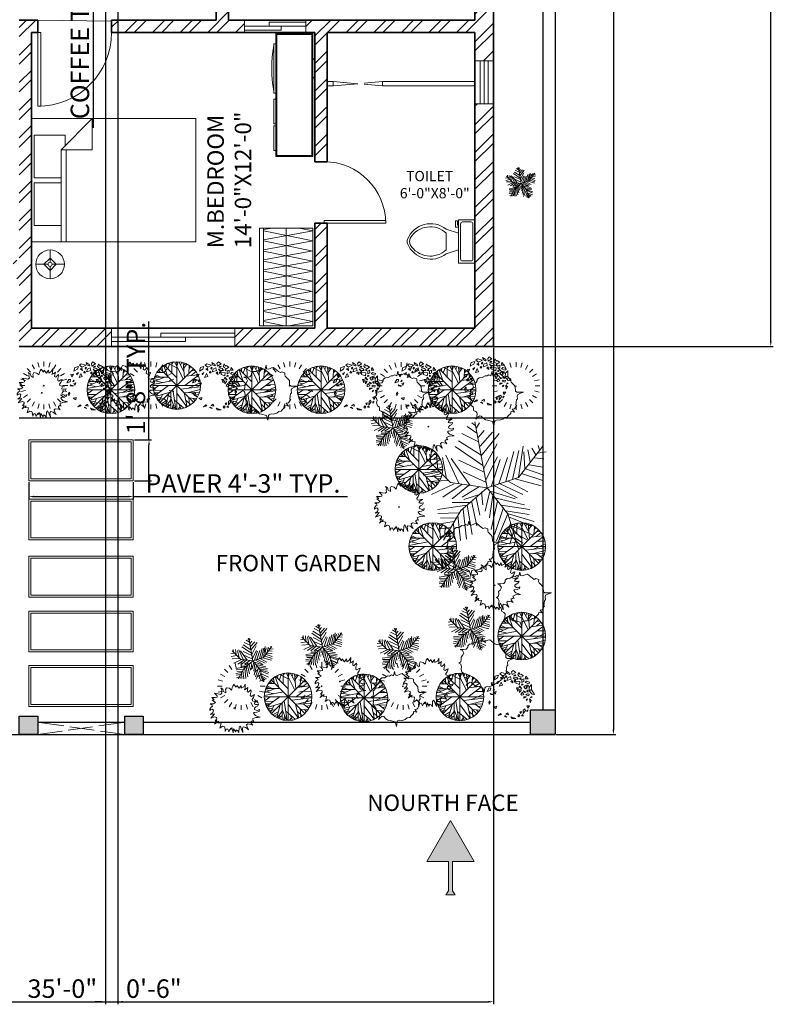
# Model space of a CAD drawing. Units: inches. Extents: x 889 to 1572, y 7262 to 8387.
# Tile 2 of 8: x 1205 to 1572, y 7262 to 7742. Entities that reach past the tile are written whole.
import ezdxf

# ---------------------------------------------------------------- set-up
doc = ezdxf.new("R2010")
doc.units = ezdxf.units.IN
doc.linetypes.add('ACAD_ISO02W100', pattern=[15, 12, -3])
for name, color, linetype, lineweight in [('A-ANNO-DIMS', 2, 'Continuous', 18), ('A-ANNO-SYMB', 7, 'Continuous', 18), ('A-ANNO-TEXT', 7, 'Continuous', 18), ('A-AREA-IDEN', 7, 'Continuous', 18), ('A-DOOR', 4, 'Continuous', 18), ('A-FIXT-HIDN', 9, 'ACAD_ISO02W100', 13), ('A-FLOR-FIXT', 9, 'Continuous', 18), ('A-FURN', 8, 'Continuous', 18), ('A-FURN-PATT', 252, 'Continuous', 13), ('A-WALL', 7, 'Continuous', 35), ('A-WALL-PATT', 252, 'Continuous', 13), ('C-SITE', 7, 'Continuous', 30), ('C-SITE-PATT', 252, 'Continuous', 13), ('L-PLNT', 94, 'Continuous', 13), ('L-PVMT', 8, 'Continuous', 18)]:
    doc.layers.add(name, color=color, linetype=linetype, lineweight=lineweight)
doc.layers.add('A-GLAZ', color=244, linetype='Continuous', lineweight=18, true_color=0x991b1e)
doc.layers.add('C-SITE-GATE', color=244, linetype='ACAD_ISO02W100', lineweight=18, true_color=0x991b1e)
doc.styles.get("Standard").update_dxf_attribs({"font": 'arial.ttf'})
doc.dimstyles.new('ISO-25', dxfattribs={"dimtxt": 9, "dimasz": 2.5, "dimexe": 1.25, "dimexo": 0.625, "dimtad": 1, "dimlunit": 3, "dimtxsty": 'Standard', "dimcen": 2.5, "dimadec": 0, "dimazin": 0, "dimtfac": 1, "dimtmove": 0, "dimatfit": 3, "dimfxl": 1, "dimarcsym": 0})

# ---------------------------------------------------------------- blocks, each defined once
blk = doc.blocks.new('*U3')
for p, q in [((0, 0), (0, -6)), ((-40, 0), (-40, -6))]:
    blk.add_line(p, q)
blk.add_lwpolyline([(0, 0), (0, 40), (-1.75, 40), (-1.75, 0)], close=True)
blk.add_arc((0, 0), 40, 90, 180)
blk = doc.blocks.new('*U4')
for p, q in [((0, 0), (0, 6)), ((40, 0), (40, 6))]:
    blk.add_line(p, q)
blk.add_lwpolyline([(0, 0), (0, -40), (1.75, -40), (1.75, 0)], close=True)
blk.add_arc((0, 0), 40, 270, 0)
blk = doc.blocks.new('*U10')
for p, q in [((9.5, -6), (9.5, -2)), ((-10, -8.5), (-8, -8.5)), ((-10, -9.5), (-10, -8.5)), ((-7, -9.5), (-10, -9.5)), ((-8, -8.5), (-8, -8)), ((-7, -8), (-7, -9.5)), ((-4, -8), (-6, -14)), ((4, -8), (6, -14)), ((4, -14), (-4, -14))]:
    blk.add_line(p, q)
blk.add_lwpolyline([(10.5, -8), (10.5, 0), (-10.5, 0), (-10.5, -8)], close=True)
for points in [[(-9.5, -2), (-9.5, -6)], [(8.5, -1), (-8.5, -1)], [(-8.5, -7), (8.5, -7)]]:
    blk.add_lwpolyline(points)
for centre, radius, start, end in [((-8.62, -1.88), 0.884, 81.8699, 188.1301), ((8.62, -1.88), 0.884, 351.8699, 98.1301), ((-8.62, -6.12), 0.884, 171.8699, 278.1301), ((8.62, -6.12), 0.884, 261.8699, 8.1301), ((3.52, -21.58), 12.17, 141.4691, 247.9714), ((4.2, -21.82), 11.33, 136.3677, 238.9468), ((-3.52, -21.58), 12.17, 292.0284, 38.5307), ((-4.2, -21.82), 11.33, 301.053, 43.6321), ((0, -27.88), 4, 245.7318, 294.2682), ((0, -29), 4, 254.8605, 285.1395)]:
    blk.add_arc(centre, radius, start, end)
blk = doc.blocks.new('Bed - Queen')
for p, q in [((0, -80.00003), (0, 0)), ((0, 0), (59.99999, 0)), ((59.99999, 0), (59.99999, -80.00003)), ((7.99999, -1.2), (28.79998, -1.2)), ((7.99999, -14.4), (7.99999, -1.2)), ((28.79998, -1.2), (28.79998, -14.4)), ((31.19999, -1.2), (51.99999, -1.2)), ((31.19999, -14.4), (31.19999, -1.2)), ((51.99999, -1.2), (51.99999, -16.4)), ((0, -14.4), (44.8, -14.4)), ((44.8, -16.8), (0, -16.8)), ((59.99999, -29.6), (44.8, -14.4)), ((44.8, -14.4), (44.8, -29.6)), ((51.99999, -16.4), (46.79936, -16.4)), ((44.8, -29.6), (59.99999, -29.6)), ((59.99999, -80.00003), (0, -80.00003))]:
    blk.add_line(p, q)
blk = doc.blocks.new('Entertainment Center')
for p, q in [((-4, 0), (-5, -1)), ((4, 0), (-4, 0)), ((5, -1), (4, 0)), ((-17, -19), (-17, -1)), ((-17, -1), (43, -1)), ((-16.5, -18.5), (-16.5, -1.5)), ((-16.5, -1.5), (42.5, -1.5)), ((42.5, -1.5), (42.5, -18.5)), ((43, -1), (43, -19)), ((43, -19), (-17, -19)), ((42.5, -18.5), (-16.5, -18.5)), ((-12, -20), (-12, -19)), ((12, -19), (12, -20)), ((15, -20), (15, -19)), ((27, -19), (27, -20)), ((28, -20), (28, -19)), ((40, -19), (40, -20)), ((12, -20), (-12, -20)), ((27, -20), (15, -20)), ((40, -20), (28, -20))]:
    blk.add_line(p, q)
blk.add_arc((0, 40), 61, 259.6111, 280.3889)
blk = doc.blocks.new('*U15')
for p, q in [((-8.737, 47.138), (-17.069, 52.711)), ((-10.186, 53.64), (-13.084, 55.962)), ((0, 0), (-10.5, 57)), ((-9.099, 51.782), (-6.563, 55.962)), ((-7.288, 39.707), (-21.778, 46.673)), ((-7.65, 43.423), (-2.578, 49.46)), ((-5.839, 35.992), (4.667, 48.067)), ((-5.114, 27.632), (10.463, 46.673)), ((-3.665, 19.273), (-27.574, 35.527)), ((-5.114, 28.097), (-24.676, 40.636)), ((-2.941, 16.486), (8.652, 37.85)), ((27, 9), (48, 36)), ((27.127, 9.056), (31.112, 35.992)), ((38.719, 34.134), (41.979, 28.561)), ((44.153, 36.456), (45.239, 32.741)), ((-31.5, 4.5), (-52.5, 25.5)), ((-48.585, 21.131), (-49.309, 29.026)), ((-43.513, 28.561), (-42.427, 15.558)), ((-38.442, 26.239), (-34.819, 7.663)), ((-35.544, 28.097), (-24.314, 3.947)), ((-1.129, 6.734), (9.014, 26.704)), ((10.101, 3.483), (17.708, 26.239)), ((16.259, 5.805), (23.142, 31.348)), ((22.055, 7.198), (27.489, 32.277)), ((31.836, 30.883), (32.561, 16.486)), ((35.096, 32.741), (37.27, 22.524)), ((40.53, 25.775), (48.862, 24.846)), ((43.791, 29.954), (51.036, 30.883)), ((-47.498, 19.737), (-55.83, 18.344)), ((-14.533, 2.09), (-30.834, 25.31)), ((-24.314, 23.917), (-2.941, 13.7)), ((3.942, 1.625), (11.187, 24.381)), ((36.183, 19.737), (48.137, 17.88)), ((-40.615, 13.7), (-55.105, 10.913)), ((-20.691, 13.7), (-1.129, 4.876)), ((0, 0), (27, 9)), ((29.662, 12.307), (48.137, 6.269)), ((33.285, 16.486), (48.862, 10.913)), ((-33.37, 6.269), (-52.207, 5.34)), ((-28.299, 3.483), (-47.86, -5.805)), ((-21.416, 3.018), (-38.079, -8.128)), ((0, 0), (-31.5, 4.5)), ((-15.982, 2.09), (-30.11, -9.521)), ((0, 0), (-22.5, -19.5)), ((-6.563, 1.161), (-21.416, -8.128)), ((0, 0), (18, -22.5)), ((6.478, 1.625), (26.04, -8.592)), ((11.187, 3.483), (30.749, -5.805)), ((18.07, 5.805), (35.096, -3.483)), ((24.229, 7.663), (46.688, 1.625)), ((-6.563, -5.805), (-19.967, -9.985)), ((-4.752, -3.483), (-3.665, -14.629)), ((2.493, -3.019), (-1.491, -20.202)), ((1.769, -2.555), (24.229, -9.521)), ((5.029, -6.27), (2.131, -25.775)), ((-17.431, -15.094), (-42.789, -18.809)), ((-15.257, -12.772), (-30.11, -12.772)), ((-17.069, -15.094), (-12.721, -40.172)), ((-13.446, -11.378), (-8.737, -32.741)), ((-9.461, -8.592), (-6.201, -23.453)), ((9.014, -11.378), (3.58, -35.992)), ((14.085, -16.951), (6.478, -40.172)), ((7.565, -9.056), (32.198, -14.629)), ((12.274, -15.094), (36.907, -18.809)), ((-24.314, -21.596), (-42.427, -22.06)), ((-22.5, -19.5), (-37.5, -45)), ((-25.038, -23.918), (-22.865, -45.281)), ((-20.691, -18.345), (-17.793, -44.352)), ((18.07, -22.524), (8.289, -45.745)), ((16.259, -19.738), (36.183, -22.989)), ((18, -22.5), (27, -52.5)), ((18.433, -22.524), (40.53, -29.026)), ((19.157, -25.311), (38.719, -33.206)), ((-28.299, -29.026), (-42.789, -31.348)), ((-26.849, -26.24), (-40.253, -25.775)), ((-29.023, -30.884), (-27.936, -43.887)), ((20.244, -30.419), (15.897, -44.816)), ((21.331, -32.741), (39.081, -40.636)), ((-30.834, -34.135), (-42.427, -35.528)), ((-34.457, -39.708), (-40.978, -42.494)), ((-32.646, -36.921), (-31.921, -44.352)), ((22.78, -37.85), (19.519, -48.532)), ((22.78, -38.314), (34.372, -44.816)), ((24.591, -45.745), (23.142, -50.854)), ((24.591, -43.423), (30.749, -47.603)), ((26.764, -49.925), (28.213, -50.854))]:
    blk.add_line(p, q)
blk = doc.blocks.new('*U14')
for points in [[(-5.78, 9.75), (-7.54, 9.23), (-8.01, 7.5), (-6.26, 8.45)], [(-4.43, 11.05), (-5.18, 10.36), (-3.96, 9.49), (-2.07, 10.36)], [(-2, 11.66), (-1.6, 10.62), (-0.52, 10.1), (-0.18, 10.62), (-0.79, 10.96)], [(1.24, 12), (0.56, 11.31), (0.76, 10.01), (2.52, 11.05)], [(2.59, 9.93), (1.84, 9.75), (1.64, 9.23), (2.32, 9.41)], [(4.14, 11.14), (3.6, 10.01), (4, 9.23), (5.22, 8.71), (6.3, 9.41), (5.08, 10.19), (4.61, 10.01)], [(-8.14, 6.03), (-9.36, 5.95), (-9.02, 4.73)], [(-5.78, 6.81), (-6.66, 6.21), (-6.52, 5.69)], [(-4.57, 6.38), (-5.45, 4.47), (-3.89, 4.82)], [(-4.84, 8.63), (-3.83, 7.85), (-4.03, 8.97)], [(-2.88, 7.5), (-3.15, 6.64), (-2.27, 6.72)], [(-1.94, 9.49), (-2.48, 8.97), (-2.27, 8.54), (-1.8, 9.06)], [(0.02, 9.06), (-1.33, 8.54), (-1.73, 7.16), (0.29, 7.76)], [(0.76, 7.16), (0.09, 6.46), (1.1, 5.95)], [(1.37, 8.54), (3.13, 8.8), (3.8, 7.85), (1.91, 7.76)], [(1.71, 6.29), (1.71, 7.07), (2.65, 7.5), (2.11, 6.9)], [(2.52, 6.81), (2.52, 5.86), (4.41, 5.17), (4.61, 6.72)], [(4.61, 8.28), (4.54, 7.76), (4.95, 7.59), (4.95, 8.28)], [(5.49, 5.51), (5.42, 4.82), (6.16, 5.08)], [(6.43, 7.94), (5.49, 7.68), (5.56, 6.21), (6.5, 6.64)], [(8.12, 4.99), (7.11, 4.65), (6.5, 4.13), (7.38, 3.09), (8.12, 3.52), (7.65, 3.87)], [(7.45, 9.32), (7.11, 7.94), (8.52, 7.94)], [(7.85, 6.81), (7.18, 6.21), (9, 5.51), (9.33, 6.38)], [(10.28, 5.17), (9.2, 4.04), (9, 2.31), (10.48, 0.49), (11.76, 0.41), (10.35, 2.48), (9.33, 2.4), (10.28, 2.83)], [(-11.32, 1.79), (-9.83, 2.31), (-9.63, 3.44), (-10.44, 3.52)], [(-8.21, 0.41), (-9.43, 0.32), (-9.83, 0.84)], [(-8.21, 3.09), (-8.48, 2.31), (-7.87, 2.57)], [(-7, 1.79), (-7.94, 1.53), (-7.47, 0.49)], [(3.53, 1.88), (2.86, 3.52), (3.8, 3.52)], [(4.41, 4.56), (4.27, 3.7), (5.49, 3.26)], [(4.27, 2.74), (5.29, 2.66), (4.41, 1.27)], [(5.83, 1.53), (5.02, 0.41), (5.49, -0.02), (6.5, 0.41)], [(7.51, 1.71), (6.91, 1.27), (6.23, 2.14)], [(8.12, 0.75), (7.51, 0.15), (8.93, -0.28), (9.13, 0.49)], [(8.19, 2.57), (7.92, 2.05), (8.66, 1.53)], [(8.73, 4.73), (8.19, 4.56), (8.39, 3.87), (8.59, 4.04)], [(-10.03, -2.71), (-10.64, -3.31), (-10.44, -4.44), (-9.9, -3.49)], [(7.78, -0.8), (6.43, -1.5), (6.43, -0.72)], [(8.32, -1.75), (7.98, -2.53), (7.58, -2.1)], [(9.33, -1.75), (9.54, -3.74), (10.14, -2.53)], [(10.08, -0.63), (9.74, -1.32), (10.48, -0.89)], [(-8.28, -5.73), (-6.79, -5.3), (-7, -6.51)], [(-4.84, -8.85), (-4.43, -9.45), (-5.99, -9.8)], [(-2.34, -9.2), (-1.26, -8.5), (-0.99, -9.54)], [(4.07, -9.45), (3.53, -9.97), (4.07, -10.58), (4.61, -9.89)], [(5.29, -7.98), (4.61, -8.16), (5.02, -8.94)], [(6.03, -9.45), (5.42, -9.97), (6.16, -10.15)], [(6.1, -8.94), (6.16, -7.21), (6.91, -6.69), (7.24, -7.38)], [(8.05, -8.07), (8.59, -7.12), (7.92, -7.55)], [(9.33, -5.13), (8.46, -6.25), (7.98, -5.22)], [(-2.54, -10.06), (-3.02, -10.23), (-1.8, -10.67)], [(0.22, -10.58), (0.83, -11.27), (2.59, -11.36)]]:
    blk.add_lwpolyline(points, close=True)
blk = doc.blocks.new('*U16')
for p, q in [((-25.024, 42.079), (-31.077, 52.563)), ((-13.435, 46.72), (-16.606, 58.557)), ((-1.077, 60.601), (-1.077, 48.601)), ((11.28, 46.72), (14.452, 58.557)), ((22.87, 42.079), (28.923, 52.563)), ((-42.564, 24.554), (-53.039, 30.601)), ((-34.93, 34.454), (-43.503, 43.028)), ((32.776, 34.454), (41.349, 43.028)), ((40.409, 24.554), (50.884, 30.601)), ((-61.077, 0.601), (-49.077, 0.601)), ((-47.5, 13.04), (-59.033, 16.131)), ((45.346, 13.04), (56.878, 16.131)), ((58.923, 0.601), (46.923, 0.601)), ((-47.5, -11.837), (-59.033, -14.928)), ((-42.564, -23.351), (-53.039, -29.399)), ((40.409, -23.351), (50.884, -29.399)), ((45.346, -11.837), (56.878, -14.928)), ((-34.93, -33.251), (-43.503, -41.825)), ((-25.024, -40.876), (-31.077, -51.36)), ((-13.435, -45.517), (-16.606, -57.354)), ((-1.077, -59.399), (-1.077, -47.399)), ((11.28, -45.517), (14.452, -57.354)), ((22.87, -40.876), (28.923, -51.36)), ((32.776, -33.251), (41.349, -41.825))]:
    blk.add_line(p, q)
blk.add_lwpolyline([(-1.908, 0.978), (-2.67, -0.978), (0, 0)], close=True)
blk = doc.blocks.new('*U17')
for p, q in [((-32.6092, 50.4264), (-23.2782, 23.5674)), ((-31.2008, 51.1035), (-0.2149, 20.1818)), ((-26.4472, 46.5894), (-26.2712, 53.8116)), ((-22.0458, 42.0753), (-16.5881, 57.6486)), ((-21.1656, 55.8436), (-0.0388, 45.0094)), ((-12.5388, 54.9406), (-7.9613, 59.4546)), ((-12.3627, 32.1443), (-12.5388, 58.7776)), ((-5.3205, 59.6806), (16.5105, 16.7963)), ((2.426, 54.9406), (-1.4472, 59.9056)), ((0, 59.9996), (0, -60)), ((0.4894, 48.6208), (3.6584, 59.6806)), ((18.2711, 35.5298), (5.419, 59.6806)), ((9.8203, 51.5549), (12.8133, 58.5516)), ((19.6795, 19.5047), (16.3344, 57.6486)), ((17.0387, 51.1035), (23.2006, 55.1666)), ((17.7429, 43.6552), (25.4894, 54.2636)), ((31.6513, 50.8778), (30.2429, 30.5643)), ((-53.2078, 27.4044), (-40.1797, 20.859)), ((-49.8627, 32.8214), (-32.7853, 32.8214)), ((-45.8134, 38.2383), (-40.5318, 33.0471)), ((-43.8768, 36.4326), (-44.405, 40.2696)), ((42, 42), (-42, -42)), ((42, -42), (-42, 42)), ((-40.1797, 44.558), (-36.4825, 43.2038)), ((-37.0107, 47.0408), (-35.25, 35.5298)), ((54.3626, 25.3731), (20.9119, 0.3198)), ((23.3767, 23.3417), (53.3063, 27.4044)), ((31.1232, 42.5267), (35.8767, 48.1693)), ((36.2288, 25.1474), (48.9049, 35.0784)), ((37.1091, 37.1098), (46.6161, 37.5612)), ((-59.7219, 2.8025), (-12.0106, 12.0565)), ((-32.2571, 20.6333), (-59.1937, 9.348)), ((-58.6656, 12.7336), (-35.9543, 7.5424)), ((-57.081, 17.9248), (-47.0458, 14.7649)), ((-56.0247, 20.859), (-20.8134, 20.859)), ((-54.7923, 24.4702), (-47.75, 21.0847)), ((-54.6162, -24.7335), (-20.2853, 0.0941)), ((29.3626, -6.6771), (59.4682, 7.091)), ((38.5175, 13.4107), (58.2359, 13.6364)), ((-60, 0), (60, 0)), ((-59.7219, -4.8714), (-54.2641, -6.6771)), ((-45.2853, -0.1316), (-59.0177, -10.0627)), ((-58.4895, -12.3197), (-36.4825, -11.6426)), ((-57.081, -18.4138), (-45.2853, -17.9624)), ((-52.6797, -18.188), (-55.4966, -22.0251)), ((-53.2078, -27.442), (-16.7641, -16.6081)), ((-47.2219, -19.3166), (-50.2148, -26.3135)), ((-35.9543, -22.4765), (-44.0529, -40.5329)), ((-19.9331, -20.2194), (-28.5599, -52.721)), ((-14.8275, -15.0282), (-14.6515, -57.6865)), ((-10.074, -10.0627), (-2.5036, -59.7178)), ((-0.0388, -19.0909), (25.8415, -53.8495)), ((9.2922, -9.1598), (59.6443, -2.8401)), ((18.6232, -18.6394), (26.7218, -53.3981)), ((18.7992, -18.6394), (57.3556, -17.2853)), ((26.3697, -18.4138), (58.9401, -9.8369)), ((38.1654, -18.188), (52.426, -29.0219)), ((45.9119, -24.0564), (55.595, -22.2508)), ((-38.9472, -29.0219), (-51.4472, -30.6018)), ((-46.5177, -30.1504), (-49.5106, -33.536)), ((-32.4331, -32.4075), (-48.1021, -35.5674)), ((-43.7008, -34.6645), (-46.6937, -37.373)), ((-24.6867, -37.8244), (-38.7712, -45.7241)), ((-26.2712, -43.9185), (-34.7219, -48.6583)), ((-14.6515, -36.2445), (-27.6797, -52.9467)), ((-14.6515, -47.3041), (-25.0388, -54.3009)), ((-21.5177, -45.4984), (-19.9331, -56.1065)), ((-14.6515, -32.1818), (-3.912, -59.4922)), ((-8.4895, -47.5298), (-11.4825, -58.5893)), ((-6.2008, -36.2445), (17.919, -57.0094)), ((5.9471, -46.6269), (10.5246, -58.5893)), ((22.8485, -36.4702), (35.3485, -48.4326)), ((24.7852, -44.8213), (23.0246, -54.978)), ((30.419, -30.1504), (32.3556, -50.0125)), ((31.4753, -31.279), (49.6091, -33.3103)), ((41.5105, -32.6332), (46.088, -38.0501)), ((-6.3768, -52.721), (-9.3698, -58.815)), ((8.4119, -53.1724), (3.8344, -59.4922))]:
    blk.add_line(p, q)
blk.add_circle((0, 0), 60)
blk = doc.blocks.new('*U18')
blk.add_lwpolyline([(-4.577, 66.508), (-7.629, 55.26), (-12.588, 57.705), (-17.165, 54.771), (-22.124, 55.26), (-29.372, 50.859), (-36.619, 50.37), (-41.578, 45.968), (-41.578, 42.056), (-45.393, 37.655), (-52.259, 36.677), (-60.651, 36.677), (-54.929, 33.743), (-51.115, 27.385), (-54.548, 21.028), (-58.362, 17.116), (-57.599, 11.248), (-58.744, 5.379), (-63.703, 2.445), (-59.125, 0), (-56.837, -6.846), (-58.362, -13.204), (-56.455, -20.539), (-52.259, -23.473), (-51.115, -27.386), (-51.115, -32.276), (-45.011, -35.21), (-41.96, -39.122), (-42.723, -47.925), (-45.393, -54.282), (-40.434, -49.392), (-35.475, -45.969), (-31.66, -46.947), (-27.083, -51.837), (-21.361, -56.238), (-16.021, -56.727), (-3.433, -60.151), (0, -71.887), (1.526, -60.151), (3.052, -58.194), (8.392, -56.238), (14.114, -56.727), (22.506, -54.282), (27.465, -50.37), (33.95, -49.392), (37.002, -44.991), (42.723, -39.611), (43.105, -35.699), (45.012, -34.721), (51.878, -36.188), (46.157, -29.342), (51.878, -28.364), (53.785, -25.919), (56.074, -21.517), (57.6, -20.539), (55.693, -18.094), (57.219, -5.868), (59.889, -2.934), (58.744, 3.423), (60.27, 7.824), (67.137, 11.248), (74.766, 14.182), (67.899, 13.693), (58.363, 13.693), (54.93, 16.627), (54.167, 27.874), (50.353, 32.276), (43.868, 39.122), (42.723, 42.545), (43.105, 47.436), (35.476, 49.881), (31.661, 47.925), (27.084, 50.859), (14.496, 61.128), (9.155, 59.661), (2.289, 56.727), (-3.051, 57.705)], close=True)
blk = doc.blocks.new('*U19')
for points in [[(0, 60.64), (-3.051, 56.238), (-4.196, 52.815), (-5.34, 47.925), (-6.103, 45.969), (-11.062, 50.859), (-18.691, 52.326), (-20.98, 47.436), (-20.217, 43.524), (-20.598, 39.611), (-25.939, 43.035), (-27.846, 49.392), (-33.186, 52.326), (-30.516, 47.436), (-31.279, 43.035), (-30.135, 38.144), (-33.568, 35.21), (-40.815, 36.677), (-49.208, 38.144), (-46.919, 36.677), (-42.341, 31.787), (-42.341, 28.364), (-46.537, 27.386), (-55.692, 27.386), (-49.97, 22.006), (-54.548, 21.028), (-46.156, 14.671), (-51.496, 11.248), (-59.888, 11.248), (-55.692, 8.803), (-53.785, 5.38), (-57.218, 3.423), (-60.651, -1.467), (-61.033, -4.89), (-59.125, -3.423), (-54.548, -1.467), (-51.496, -4.401), (-53.022, -10.269), (-59.125, -15.16), (-49.208, -13.204), (-58.362, -24.451), (-48.445, -21.028), (-43.486, -22.495), (-43.104, -25.918), (-47.3, -31.298), (-43.104, -30.32), (-48.445, -39.611), (-38.527, -31.787), (-40.815, -36.188), (-32.423, -37.166), (-33.568, -43.523), (-35.475, -49.392), (-28.609, -44.99), (-23.65, -46.457), (-22.124, -51.837), (-21.743, -57.705), (-19.073, -52.326), (-15.639, -51.837), (-12.588, -58.683), (-11.062, -54.771), (-6.866, -49.392), (-6.866, -53.304), (-4.959, -48.414), (-1.907, -61.617), (-1.144, -51.348), (4.578, -59.172), (5.341, -54.282), (9.918, -56.727), (12.207, -60.639), (12.97, -47.925), (14.877, -44.501), (17.547, -47.436), (19.455, -52.815), (22.888, -60.639), (21.743, -49.392), (23.65, -46.457), (29.754, -47.925), (35.094, -52.326), (37.001, -53.793), (33.187, -46.457), (32.042, -41.567), (35.094, -39.122), (43.868, -40.589), (47.682, -42.056), (43.105, -36.188), (43.105, -33.743), (46.538, -31.298), (50.352, -32.765), (46.919, -26.407), (55.693, -22.495), (60.652, -22.984), (66.374, -22.006), (59.889, -20.05), (54.167, -18.094), (51.878, -15.649), (49.589, -12.225), (51.497, -10.269), (57.981, -9.78), (63.322, -7.335), (64.466, -2.934)], [(64.848, -2.934), (59.507, -5.379), (56.456, -4.401), (51.878, -2.445), (52.26, 0.978), (55.311, 3.912), (59.889, 5.869), (62.94, 11.248), (58.363, 10.27), (54.548, 10.27), (51.115, 11.248), (53.785, 15.649), (57.981, 18.094), (60.652, 19.561), (56.074, 19.561), (51.115, 17.605), (46.538, 19.072), (46.156, 22.496), (49.589, 27.386), (52.26, 34.721), (49.589, 33.743), (44.249, 30.32), (41.197, 32.276), (41.579, 37.655), (43.868, 42.546), (43.105, 46.947), (40.053, 44.013), (36.238, 40.589), (33.568, 42.057), (33.95, 45.969), (35.476, 52.815), (31.28, 49.392), (26.702, 46.947), (28.228, 50.859), (28.609, 61.129), (24.795, 54.282), (18.692, 50.859), (17.929, 57.706), (12.97, 50.859), (7.248, 57.706), (5.341, 53.304), (0, 60.64)]]:
    blk.add_lwpolyline(points)
blk.add_lwpolyline([(0.382, 1.956), (0, 0), (1.907, 0.489), (2.289, 1.467)], close=True)
blk = doc.blocks.new('Lamp - Table')
for p, q in [((0, 7), (0, 1)), ((-1, 0), (-7, 0)), ((0, 3), (-3, 0)), ((-3, 0), (0, -3)), ((3, 0), (0, 3)), ((0, -3), (3, 0)), ((1, 0), (7, 0)), ((0, -1), (0, -7))]:
    blk.add_line(p, q)
for radius in [7, 1]:
    blk.add_circle((0, 0), radius)
blk = doc.blocks.new('*D29')
at = {"layer": 'A-ANNO-DIMS', "color": 0, "lineweight": -2, "transparency": 16777216}
for p, q in [((1466.67, 8272.73), (1495.73, 8272.73)), ((1494.48, 8270.23), (1494.48, 7396.23)), ((1466.67, 7393.73), (1495.73, 7393.73))]:
    blk.add_line(p, q, dxfattribs=at)
at = {"layer": 'A-ANNO-DIMS', "color": 0, "transparency": 16777216}
for points in [[(1494.06, 8270.23), (1494.9, 8270.23), (1494.48, 8272.73)], [(1494.06, 7396.23), (1494.9, 7396.23), (1494.48, 7393.73)]]:
    blk.add_solid(points, dxfattribs=at)
at = {"layer": 'Defpoints', "color": 0, "transparency": 16777216}
for p in [(1466.05, 8272.73), (1466.05, 7393.73), (1494.48, 7393.73)]:
    blk.add_point(p, dxfattribs=at)
at = {"layer": 'A-ANNO-DIMS', "color": 0, "transparency": 16777216, "insert": (1489.26, 7833.23), "char_height": 9, "attachment_point": 5, "rotation": 90}
blk.add_mtext('73\'-3"', dxfattribs=at)
blk = doc.blocks.new('WALK-STEPPING-SLAB')
for points in [[(0, 0), (50.92, 0), (50.92, 19.94), (0, 19.94)], [(1, 1), (49.92, 1), (49.92, 18.94), (1, 18.94)]]:
    blk.add_lwpolyline(points, close=True)
blk = doc.blocks.new('GLAZ-VENT-21IN')
for p, q in [((0, 4), (21, 4)), ((0, 2), (21, 2)), ((0, 0), (21, 0))]:
    blk.add_line(p, q)
blk = doc.blocks.new('GLAZ-SLIDER-60IN')
for p, q in [((0, 60), (0, 24)), ((2, 60), (2, 0)), ((2, 36), (4, 36)), ((4, 36), (4, 0)), ((2, 24), (0, 24))]:
    blk.add_line(p, q)
blk = doc.blocks.new('GLAZ-SLIDER-30IN')
for p, q in [((0, 30), (0, 12)), ((2, 30), (2, 0)), ((4, 18), (2, 18)), ((4, 18), (4, 0)), ((2, 12), (0, 12))]:
    blk.add_line(p, q)
blk = doc.blocks.new('*D51')
at = {"layer": 'A-ANNO-DIMS', "color": 0, "lineweight": -2, "transparency": 16777216}
for p, q in [((1209.71, 7516.66), (1209.71, 7508.4)), ((1260.62, 7516.66), (1260.62, 7508.4)), ((1212.21, 7509.65), (1258.12, 7509.65)), ((1260.62, 7509.65), (1364.9, 7509.65))]:
    blk.add_line(p, q, dxfattribs=at)
at = {"layer": 'A-ANNO-DIMS', "color": 0, "transparency": 16777216}
for points in [[(1212.21, 7510.07), (1212.21, 7509.23), (1209.71, 7509.65)], [(1258.12, 7510.07), (1258.12, 7509.23), (1260.62, 7509.65)]]:
    blk.add_solid(points, dxfattribs=at)
at = {"layer": 'Defpoints', "color": 0, "transparency": 16777216}
for p in [(1209.71, 7517.29), (1260.62, 7517.29), (1260.62, 7509.65)]:
    blk.add_point(p, dxfattribs=at)
at = {"layer": 'A-ANNO-DIMS', "color": 0, "transparency": 16777216, "insert": (1314.01, 7514.87), "char_height": 9, "attachment_point": 5}
blk.add_mtext('PAVER 4\'-3" TYP.', dxfattribs=at)
blk = doc.blocks.new('*D52')
at = {"layer": 'A-ANNO-DIMS', "color": 0, "lineweight": -2, "transparency": 16777216}
for p, q in [((1268.26, 7537.22), (1268.26, 7594.99)), ((1261.25, 7537.22), (1269.51, 7537.22)), ((1268.26, 7519.79), (1268.26, 7534.72)), ((1261.25, 7517.29), (1269.51, 7517.29))]:
    blk.add_line(p, q, dxfattribs=at)
at = {"layer": 'A-ANNO-DIMS', "color": 0, "transparency": 16777216}
for points in [[(1267.85, 7534.72), (1268.68, 7534.72), (1268.26, 7537.22)], [(1267.85, 7519.79), (1268.68, 7519.79), (1268.26, 7517.29)]]:
    blk.add_solid(points, dxfattribs=at)
at = {"layer": 'Defpoints', "color": 0, "transparency": 16777216}
for p in [(1260.62, 7537.22), (1268.26, 7537.22), (1260.62, 7517.29)]:
    blk.add_point(p, dxfattribs=at)
at = {"layer": 'A-ANNO-DIMS', "color": 0, "transparency": 16777216, "insert": (1263.04, 7567.35), "char_height": 9, "attachment_point": 5, "rotation": 90}
blk.add_mtext('1\'-8" TYP.', dxfattribs=at)
blk = doc.blocks.new('*D67')
at = {"layer": 'A-ANNO-DIMS', "color": 0, "lineweight": -2, "transparency": 16777216}
for p, q in [((1232.68, 7874.55), (1242.3, 7874.55)), ((1241.05, 7872.05), (1241.05, 7817.05)), ((1232.68, 7814.55), (1242.3, 7814.55)), ((1241.05, 7814.55), (1241.05, 7689.17))]:
    blk.add_line(p, q, dxfattribs=at)
at = {"layer": 'A-ANNO-DIMS', "color": 0, "transparency": 16777216}
for points in [[(1240.64, 7872.05), (1241.47, 7872.05), (1241.05, 7874.55)], [(1240.64, 7817.05), (1241.47, 7817.05), (1241.05, 7814.55)]]:
    blk.add_solid(points, dxfattribs=at)
at = {"layer": 'Defpoints', "color": 0, "transparency": 16777216}
for p in [(1232.05, 7874.55), (1232.05, 7814.55), (1241.05, 7814.55)]:
    blk.add_point(p, dxfattribs=at)
at = {"layer": 'A-ANNO-DIMS', "color": 0, "transparency": 16777216, "insert": (1235.77, 7750.61), "char_height": 9, "attachment_point": 5, "rotation": 90}
blk.add_mtext('COFFEE TABLE 5\'-0"', dxfattribs=at)
blk = doc.blocks.new('*D69')
at = {"layer": 'A-ANNO-DIMS', "color": 0, "lineweight": -2, "transparency": 16777216}
for p, q in [((1016.05, 7615.11), (1016.05, 7262.35)), ((1436.05, 7582.11), (1436.05, 7262.35)), ((1018.55, 7263.6), (1433.55, 7263.6))]:
    blk.add_line(p, q, dxfattribs=at)
at = {"layer": 'A-ANNO-DIMS', "color": 0, "transparency": 16777216}
for points in [[(1018.55, 7264.02), (1018.55, 7263.19), (1016.05, 7263.6)], [(1433.55, 7264.02), (1433.55, 7263.19), (1436.05, 7263.6)]]:
    blk.add_solid(points, dxfattribs=at)
at = {"layer": 'Defpoints', "color": 0, "transparency": 16777216}
for p in [(1016.05, 7615.73), (1436.05, 7582.73), (1436.05, 7263.6)]:
    blk.add_point(p, dxfattribs=at)
at = {"layer": 'A-ANNO-DIMS', "color": 0, "transparency": 16777216, "insert": (1226.05, 7268.83), "char_height": 9, "attachment_point": 5}
blk.add_mtext('35\'-0"', dxfattribs=at)
blk = doc.blocks.new('*D70')
at = {"layer": 'A-ANNO-DIMS', "color": 0, "lineweight": -2, "transparency": 16777216}
for p, q in [((1436.67, 8272.73), (1572.38, 8272.73)), ((1571.13, 7585.23), (1571.13, 8270.23)), ((1436.67, 7582.73), (1572.38, 7582.73))]:
    blk.add_line(p, q, dxfattribs=at)
at = {"layer": 'A-ANNO-DIMS', "color": 0, "transparency": 16777216}
for points in [[(1570.71, 8270.23), (1571.54, 8270.23), (1571.13, 8272.73)], [(1570.71, 7585.23), (1571.54, 7585.23), (1571.13, 7582.73)]]:
    blk.add_solid(points, dxfattribs=at)
at = {"layer": 'Defpoints', "color": 0, "transparency": 16777216}
for p in [(1436.05, 8272.73), (1571.13, 8272.73), (1436.05, 7582.73)]:
    blk.add_point(p, dxfattribs=at)
at = {"layer": 'A-ANNO-DIMS', "color": 0, "transparency": 16777216, "insert": (1565.91, 7927.73), "char_height": 9, "attachment_point": 5, "rotation": 90}
blk.add_mtext('57\'-6"', dxfattribs=at)
blk = doc.blocks.new('*D74')
at = {"layer": 'A-ANNO-DIMS', "color": 0, "lineweight": -2, "transparency": 16777216}
for p, q in [((1247.05, 8161.11), (1247.05, 7262.35)), ((1253.05, 8161.11), (1253.05, 7262.35)), ((1244.55, 7263.6), (1242.05, 7263.6)), ((1247.05, 7263.6), (1253.05, 7263.6)), ((1255.55, 7263.6), (1283.22, 7263.6))]:
    blk.add_line(p, q, dxfattribs=at)
at = {"layer": 'A-ANNO-DIMS', "color": 0, "transparency": 16777216}
for points in [[(1244.55, 7264.02), (1244.55, 7263.19), (1247.05, 7263.6)], [(1255.55, 7264.02), (1255.55, 7263.19), (1253.05, 7263.6)]]:
    blk.add_solid(points, dxfattribs=at)
at = {"layer": 'Defpoints', "color": 0, "transparency": 16777216}
for p in [(1247.05, 8161.73), (1253.05, 8161.73), (1253.05, 7263.6)]:
    blk.add_point(p, dxfattribs=at)
at = {"layer": 'A-ANNO-DIMS', "color": 0, "transparency": 16777216, "insert": (1270.64, 7268.82), "char_height": 9, "attachment_point": 5}
blk.add_mtext('0\'-6"', dxfattribs=at)

msp = doc.modelspace()

# ---------------------------------------------------------------- hatches: boundary and pattern name
at = {"layer": 'A-ANNO-SYMB'}
h = msp.add_hatch(color=256, dxfattribs=at)
h.dxf.hatch_style = 1
h.paths.add_polyline_path([(1415.135, 7351.849), (1403.632, 7331.925), (1414.135, 7331.925), (1414.135, 7317.604), (1412.866, 7315.604), (1417.406, 7315.604), (1416.135, 7317.604), (1416.135, 7331.925), (1426.638, 7331.925)])
at = {"layer": 'A-FURN-PATT'}
h = msp.add_hatch(dxfattribs=at)
h.set_pattern_fill('ANSI31', color=256, scale=1.523476, angle=-34.69827, style=0)
h.paths.add_polyline_path([(1324.049, 7592.731), (1348.049, 7592.731), (1348.049, 7640.438), (1324.049, 7640.438)])
h = msp.add_hatch(dxfattribs=at)
h.set_pattern_fill('ANSI31', color=256, scale=1.5169374, angle=123.42338, style=0)
h.paths.add_polyline_path([(1324.049, 7592.731), (1348.049, 7592.731), (1348.049, 7640.438), (1324.049, 7640.438)])
at = {"layer": 'A-WALL-PATT'}
h = msp.add_hatch(dxfattribs=at)
h.set_pattern_fill('ANSI32', color=256)
h.paths.add_polyline_path([(1166.049, 7624.731), (1163.049, 7624.731), (1163.049, 7774.731), (1154.049, 7774.731), (1154.049, 7768.731), (1157.049, 7768.731), (1157.049, 7624.731), (1106.049, 7624.731), (1106.049, 7615.731), (1166.049, 7615.731), (1166.049, 7618.431)])
h.paths.add_polyline_path([(1025.049, 7666.731), (1016.049, 7666.731), (1016.049, 7615.731), (1076.049, 7615.731), (1076.049, 7624.731), (1025.049, 7624.731)])
h.paths.add_polyline_path([(1025.049, 7768.731), (1118.049, 7768.731), (1118.049, 7774.731), (1025.049, 7774.731), (1025.049, 7897.731), (1115.049, 7897.731), (1115.049, 7906.731), (1109.049, 7906.731), (1109.049, 7903.731), (1025.049, 7903.731), (1025.049, 7923.231), (1016.049, 7923.231), (1016.049, 7726.731), (1025.049, 7726.731)])
h.paths.add_polyline_path([(1436.049, 7897.731), (1427.049, 7897.731), (1427.049, 7883.374), (1436.049, 7883.374)])
h.paths.add_polyline_path([(1436.049, 7853.374), (1427.049, 7853.374), (1427.049, 7843.731), (1415.049, 7843.731), (1415.049, 7837.731), (1427.049, 7837.731), (1427.049, 7831.731), (1436.049, 7831.731)])
h.paths.add_polyline_path([(1436.049, 8010.183), (1427.049, 8010.183), (1427.049, 7970.456), (1370.049, 7970.456), (1370.049, 7963.731), (1427.049, 7963.731), (1427.049, 7957.731), (1436.049, 7957.731)])
h.paths.add_polyline_path([(1436.049, 7747.731), (1427.049, 7747.731), (1427.049, 7741.731), (1344.721, 7741.731), (1344.721, 7735.731), (1349.049, 7735.731), (1349.049, 7672.731), (1355.049, 7672.731), (1355.049, 7735.731), (1427.049, 7735.731), (1427.049, 7721.931), (1436.049, 7721.931)])
h.paths.add_polyline_path([(1436.049, 7700.931), (1427.049, 7700.931), (1427.049, 7591.731), (1355.049, 7591.731), (1355.049, 7642.731), (1349.049, 7642.731), (1349.049, 7591.731), (1310.049, 7591.731), (1310.049, 7582.731), (1436.049, 7582.731)])
h.paths.add_polyline_path([(1392.42, 8272.731), (1331.049, 8272.731), (1331.049, 8263.731), (1349.049, 8263.731), (1349.049, 8224.731), (1355.049, 8224.731), (1355.049, 8263.731), (1392.42, 8263.731)])
h.paths.add_polyline_path([(1271.049, 8272.731), (1196.736, 8272.731), (1196.736, 8263.731), (1247.049, 8263.731), (1247.049, 8203.731), (1244.049, 8203.731), (1244.049, 8197.731), (1247.049, 8197.731), (1247.049, 8161.731), (1253.049, 8161.731), (1253.049, 8185.731), (1295.049, 8185.731), (1295.049, 8191.731), (1253.049, 8191.731), (1253.049, 8263.731), (1271.049, 8263.731)])
h.paths.add_polyline_path([(1175.736, 8272.731), (1102.037, 8272.731), (1102.037, 8263.731), (1157.049, 8263.731), (1157.049, 8158.731), (1163.049, 8158.731), (1163.049, 8197.731), (1214.049, 8197.731), (1214.049, 8203.731), (1163.049, 8203.731), (1163.049, 8263.731), (1175.736, 8263.731)])
h.paths.add_polyline_path([(1072.037, 8272.731), (1016.049, 8272.731), (1016.049, 8221.731), (1025.049, 8221.731), (1025.049, 8263.731), (1072.037, 8263.731)])
h.paths.add_polyline_path([(1163.049, 8122.731), (1157.049, 8122.731), (1157.049, 8119.731), (1025.049, 8119.731), (1025.049, 8161.731), (1016.049, 8161.731), (1016.049, 8071.731), (1025.049, 8071.731), (1025.049, 8113.731), (1157.049, 8113.731), (1157.049, 8110.731), (1163.049, 8110.731)])
h.paths.add_polyline_path([(1025.049, 8011.731), (1016.049, 8011.731), (1016.049, 7944.231), (1025.049, 7944.231), (1025.049, 7963.731), (1109.049, 7963.731), (1109.049, 7936.731), (1115.049, 7936.731), (1115.049, 7963.731), (1163.049, 7963.731), (1163.049, 8074.731), (1157.049, 8074.731), (1157.049, 7969.731), (1025.049, 7969.731)])
h.paths.add_polyline_path([(1314.721, 7741.731), (1307.049, 7741.731), (1307.049, 7837.731), (1319.049, 7837.731), (1319.049, 7843.731), (1307.049, 7843.731), (1307.049, 7963.731), (1310.049, 7963.731), (1310.049, 7970.456), (1301.049, 7970.456), (1301.049, 7837.731), (1301.049, 7741.731), (1250.049, 7741.731), (1250.049, 7735.731), (1314.721, 7735.731)])
h.paths.add_polyline_path([(1211.049, 7735.731), (1214.049, 7735.731), (1214.049, 7741.731), (1205.049, 7741.731), (1205.049, 7624.731), (1202.049, 7624.731), (1202.049, 7615.731), (1205.049, 7615.731), (1205.049, 7582.731), (1250.049, 7582.731), (1250.049, 7591.731), (1211.049, 7591.731)])
h.paths.add_polyline_path([(1436.049, 8260.718), (1427.049, 8260.718), (1427.049, 8191.731), (1355.049, 8191.731), (1355.049, 8194.731), (1349.049, 8194.731), (1349.049, 8191.731), (1343.049, 8191.731), (1343.049, 8185.731), (1427.049, 8185.731), (1427.049, 8070.183), (1436.049, 8070.183)])
at = {"layer": 'C-SITE-PATT'}
h = msp.add_hatch(color=256, dxfattribs=at)
h.dxf.hatch_style = 1
h.paths.add_polyline_path([(1214.049, 7402.731), (1205.049, 7402.731), (1205.049, 7393.731), (1214.049, 7393.731)])
h.paths.add_polyline_path([(1265.481, 7402.731), (1256.481, 7402.731), (1256.481, 7393.731), (1265.481, 7393.731)])
h.paths.add_polyline_path([(998.049, 7405.731), (986.049, 7405.731), (986.049, 7393.731), (998.049, 7393.731)])
h = msp.add_hatch(color=256, dxfattribs=at)
h.dxf.hatch_style = 1
h.paths.add_polyline_path([(1466.049, 7405.731), (1454.049, 7405.731), (1454.049, 7393.731), (1466.049, 7393.731)])

# ---------------------------------------------------------------- linework, layer by layer
at = {"layer": 'A-ANNO-SYMB'}
for p, q in [((1414.135, 7331.925), (1414.135, 7317.604)), ((1416.135, 7331.925), (1416.135, 7317.604)), ((1412.866, 7315.604), (1414.135, 7317.604)), ((1412.866, 7315.604), (1417.406, 7315.604)), ((1417.406, 7315.604), (1416.135, 7317.604))]:
    msp.add_line(p, q, dxfattribs=at)
msp.add_lwpolyline([(1416.135, 7331.925), (1426.638, 7331.925), (1415.135, 7351.849), (1403.632, 7331.925), (1414.135, 7331.925)], dxfattribs=at)
at = {"layer": 'A-DOOR'}
msp.add_line((1214.049, 7741.731), (1250.049, 7741.131), dxfattribs=at)
at = {"layer": 'A-FIXT-HIDN'}
for p, q in [((1358.049, 7711.731), (1382.049, 7709.731)), ((1358.049, 7709.731), (1382.049, 7711.731))]:
    msp.add_line(p, q, dxfattribs=at)
at = {"layer": 'A-FLOR-FIXT'}
for p, q in [((1355.049, 7711.731), (1358.049, 7711.731)), ((1358.049, 7711.731), (1358.049, 7709.731)), ((1382.049, 7711.731), (1382.049, 7709.731)), ((1382.049, 7711.731), (1427.049, 7711.731)), ((1355.049, 7709.731), (1358.049, 7709.731)), ((1382.049, 7709.731), (1427.049, 7709.731))]:
    msp.add_line(p, q, dxfattribs=at)
at = {"layer": 'A-FURN'}
for p, q in [((1322.049, 7640.438), (1322.049, 7592.731)), ((1348.049, 7640.438), (1322.049, 7640.438)), ((1324.049, 7640.438), (1324.049, 7592.731)), ((1335.049, 7640.438), (1335.049, 7592.731)), ((1348.049, 7640.438), (1348.049, 7592.731)), ((1322.049, 7592.731), (1348.049, 7592.731))]:
    msp.add_line(p, q, dxfattribs=at)
at = {"layer": 'A-GLAZ'}
for points in [[(1314.721, 7741.731), (1344.721, 7741.731), (1344.721, 7735.731), (1314.721, 7735.731)], [(1436.049, 7721.931), (1436.049, 7700.931), (1427.049, 7700.931), (1427.049, 7721.931)], [(1310.049, 7591.731), (1310.049, 7582.731), (1250.049, 7582.731), (1250.049, 7591.731)]]:
    msp.add_lwpolyline(points, close=True, dxfattribs=at)
at = {"layer": 'A-WALL'}
for p, q in [((1436.049, 8272.731), (1436.049, 7582.731)), ((1301.049, 7837.731), (1301.049, 7741.731)), ((1307.049, 7837.731), (1307.049, 7741.731)), ((1427.049, 7837.731), (1427.049, 7741.731)), ((1205.049, 7741.731), (1214.049, 7741.731)), ((1214.049, 7735.731), (1214.049, 7741.731)), ((1250.049, 7735.731), (1250.049, 7741.731)), ((1250.049, 7741.731), (1301.049, 7741.731)), ((1307.049, 7741.731), (1427.049, 7741.731)), ((1211.049, 7735.731), (1214.049, 7735.731)), ((1211.049, 7735.731), (1211.049, 7591.731)), ((1250.049, 7735.731), (1349.049, 7735.731)), ((1349.049, 7735.731), (1349.049, 7672.731)), ((1355.049, 7735.731), (1355.049, 7672.731)), ((1355.049, 7735.731), (1427.049, 7735.731)), ((1427.049, 7735.731), (1427.049, 7591.731)), ((1349.049, 7672.731), (1355.049, 7672.731)), ((1349.049, 7642.731), (1349.049, 7591.731)), ((1349.049, 7642.731), (1355.049, 7642.731)), ((1355.049, 7642.731), (1355.049, 7591.731)), ((1211.049, 7591.731), (1349.049, 7591.731)), ((1355.049, 7591.731), (1427.049, 7591.731)), ((1205.049, 7582.731), (1436.049, 7582.731))]:
    msp.add_line(p, q, dxfattribs=at)
at = {"layer": 'C-SITE'}
for p, q in [((1466.049, 8272.731), (1466.049, 7582.731)), ((1460.049, 8266.729), (1460.049, 7582.731)), ((1436.049, 7582.731), (1466.049, 7582.731)), ((1460.049, 7582.731), (1460.049, 7405.731)), ((1466.049, 7582.731), (1466.049, 7393.731)), ((1205.049, 7547.964), (1460.049, 7547.964)), ((1214.049, 7399.731), (1256.481, 7399.731)), ((1265.481, 7399.731), (1454.049, 7399.731)), ((986.049, 7393.731), (1466.049, 7393.731))]:
    msp.add_line(p, q, dxfattribs=at)
for points in [[(1454.049, 7405.731), (1466.049, 7405.731), (1466.049, 7393.731), (1454.049, 7393.731)], [(1205.049, 7402.731), (1214.049, 7402.731), (1214.049, 7393.731), (1205.049, 7393.731)], [(1256.481, 7402.731), (1265.481, 7402.731), (1265.481, 7393.731), (1256.481, 7393.731)]]:
    msp.add_lwpolyline(points, close=True, dxfattribs=at)
at = {"layer": 'C-SITE-GATE'}
for p, q in [((1214.049, 7393.731), (1256.481, 7399.731)), ((1256.481, 7393.731), (1214.049, 7399.731))]:
    msp.add_line(p, q, dxfattribs=at)

# ---------------------------------------------------------------- block references
at = {"layer": 'A-DOOR', "xscale": 0.9, "yscale": 0.9, "zscale": 0.9}
msp.add_blockref('*U4', (1214.049, 7735.731), dxfattribs=at)
at = {"layer": 'A-DOOR', "xscale": 0.75, "yscale": 0.75, "zscale": 0.75, "rotation": 270.0000000000077}
msp.add_blockref('*U3', (1353.549, 7642.731), dxfattribs=at)
at = {"layer": 'A-FLOR-FIXT', "rotation": 270}
msp.add_blockref('*U10', (1427.049, 7633.898), dxfattribs=at)
at = {"layer": 'A-FURN'}
for name, p, rotation in [('Entertainment Center', (1349.049, 7718.207), 270), ('Bed - Queen', (1211.049, 7633.731), 90)]:
    msp.add_blockref(name, p, dxfattribs=dict(at, rotation=rotation))
msp.add_blockref('Lamp - Table', (1220.077, 7622.763), dxfattribs=at)
at = {"layer": 'A-GLAZ'}
for name, p, rotation in [('GLAZ-SLIDER-30IN', (1314.722, 7740.731), 269.9999999999963), ('GLAZ-VENT-21IN', (1433.549, 7700.931), 89.99999999999066), ('GLAZ-SLIDER-60IN', (1310.049, 7585.232), 89.9999999999985)]:
    msp.add_blockref(name, p, dxfattribs=dict(at, rotation=rotation))
at = {"layer": 'L-PLNT'}
for name, p, xscale, yscale, zscale in [('*U15', (1449.619, 7662.137), 0.137481440781912, 0.137481440781912, 0.137481440781912), ('*U16', (1217.301, 7563.658), 0.1933350602742839, 0.1933350602742839, 0.1933350602742839), ('*U17', (1249.717, 7561.68), 0.1933350602742839, 0.1933350602742839, 0.1933350602742839), ('*U19', (1258.985, 7563.406), 0.1933350602742839, 0.1933350602742839, 0.1933350602742839), ('*U16', (1269.34, 7563.658), 0.1933350602742839, 0.1933350602742839, 0.1933350602742839), ('*U17', (1281.747, 7563.722), 0.1933350602742839, 0.1933350602742839, 0.1933350602742839), ('*U17', (1318.407, 7561.68), 0.1933350602742839, 0.1933350602742839, 0.1933350602742839), ('*U18', (1326.156, 7560.745), 0.1933350602742839, 0.1933350602742839, 0.1933350602742839), ('*U16', (1337.004, 7563.658), 0.1933350602742839, 0.1933350602742839, 0.1933350602742839), ('*U17', (1352.055, 7561.68), 0.1933350602742839, 0.1933350602742839, 0.1933350602742839), ('*U16', (1391.25, 7563.433), 0.1933350602742839, 0.1933350602742839, 0.1933350602742839), ('*U17', (1415.899, 7561.68), 0.1933350602742839, 0.1933350602742839, 0.1933350602742839), ('*U16', (1447.261, 7563.433), 0.1933350602742839, 0.1933350602742839, 0.1933350602742839), ('*U19', (1215.806, 7559.992), 0.1933350602742839, 0.1933350602742839, 0.1933350602742839), ('*U18', (1390.425, 7557.822), 0.1933350602742839, 0.1933350602742839, 0.1933350602742839), ('*U18', (1436.233, 7557.822), 0.1933350602742839, 0.1933350602742839, 0.1933350602742839), ('*U15', (1387.178, 7542.996), 0.1933350602742839, 0.1933350602742839, 0.1933350602742839), ('*U19', (1404.137, 7543.545), 0.1933350602742839, 0.1933350602742839, 0.1933350602742839), ('*U15', (1432.928, 7513.915), 0.5650163262662345, 0.5650163262662345, 0.5650163262662345), ('*U17', (1399.733, 7522.891), 0.1933350602742839, 0.1933350602742839, 0.1933350602742839), ('*U19', (1389.852, 7504.425), 0.1933350602742839, 0.1933350602742839, 0.1933350602742839), ('*U17', (1406.479, 7485.308), 0.1933350602742839, 0.1933350602742839, 0.1933350602742839), ('*U18', (1424.996, 7484.812), 0.1933350602742839, 0.1933350602742839, 0.1933350602742839), ('*U17', (1449.849, 7485.308), 0.1933350602742839, 0.1933350602742839, 0.1933350602742839), ('*U15', (1417.82, 7474.046), 0.1933350602742839, 0.1933350602742839, 0.1933350602742839), ('*U19', (1436.423, 7466.259), 0.1933350602742839, 0.1933350602742839, 0.1933350602742839), ('*U18', (1449.808, 7460.035), 0.1933350602742839, 0.1933350602742839, 0.1933350602742839), ('*U15', (1424.81, 7444.963), 0.1933350602742839, 0.1933350602742839, 0.1933350602742839), ('*U17', (1449.849, 7441.689), 0.1933350602742839, 0.1933350602742839, 0.1933350602742839), ('*U15', (1352.856, 7436.308), 0.1933350602742839, 0.1933350602742839, 0.1933350602742839), ('*U15', (1390.191, 7434.503), 0.1933350602742839, 0.1933350602742839, 0.1933350602742839), ('*U15', (1318.871, 7429.591), 0.1933350602742839, 0.1933350602742839, 0.1933350602742839), ('*U18', (1431.54, 7428.1), 0.1933350602742839, 0.1933350602742839, 0.1933350602742839), ('*U16', (1313.39, 7417.239), 0.1933350602742839, 0.1933350602742839, 0.1933350602742839), ('*U16', (1352.621, 7417.239), 0.1933350602742839, 0.1933350602742839, 0.1933350602742839), ('*U19', (1360.987, 7419.398), 0.1933350602742839, 0.1933350602742839, 0.1933350602742839), ('*U16', (1392.234, 7417.239), 0.1933350602742839, 0.1933350602742839, 0.1933350602742839), ('*U19', (1403.927, 7419.058), 0.1933350602742839, 0.1933350602742839, 0.1933350602742839), ('*U17', (1336.034, 7412.183), 0.1933350602742839, 0.1933350602742839, 0.1933350602742839), ('*U18', (1388.775, 7411.611), 0.1933350602742839, 0.1933350602742839, 0.1933350602742839), ('*U17', (1419.745, 7412.043), 0.1933350602742839, 0.1933350602742839, 0.1933350602742839), ('*U17', (1372.993, 7411.598), 0.1933350602742839, 0.1933350602742839, 0.1933350602742839), ('*U19', (1309.613, 7406.456), 0.1933350602742839, 0.1933350602742839, 0.1933350602742839)]:
    msp.add_blockref(name, p, dxfattribs=dict(at, xscale=xscale, yscale=yscale, zscale=zscale))
for p in [(1432.728, 7565.66), (1239.619, 7563.228), (1300.816, 7563.228), (1369.321, 7563.228), (1399.409, 7563.228), (1444.361, 7412.898)]:
    msp.add_blockref('*U14', p, dxfattribs=at)
at = {"layer": 'L-PVMT'}
for p in [(1209.706, 7517.288), (1209.706, 7488.504), (1209.706, 7460.693), (1209.706, 7433.97), (1209.706, 7407.405)]:
    msp.add_blockref('WALK-STEPPING-SLAB', p, dxfattribs=at)

# ---------------------------------------------------------------- texts
at = {"layer": 'A-ANNO-TEXT', "insert": (1374.587, 7364.527), "char_height": 8, "attachment_point": 1}
msp.add_mtext_dynamic_manual_height_columns('NOURTH FACE', width=81.18436, gutter_width=12.5, heights=[0], dxfattribs=at)
at = {"layer": 'A-AREA-IDEN', "insert": (1296.71, 7630.59), "char_height": 8, "attachment_point": 1, "rotation": 90}
msp.add_mtext_dynamic_manual_height_columns('M.BEDROOM\\P 14\'-0"X12\'-0"', width=66.55508, gutter_width=12.5, heights=[0], dxfattribs=at)
at = {"layer": 'A-AREA-IDEN', "attachment_point": 1}
for s, width, insert, char_height in [('  TOILET\\P6\'-0"X8\'-0"', 32.40356, (1390.436, 7668.249), 5), ('FRONT GARDEN', 90.43616, (1300.789, 7481.245), 8)]:
    msp.add_mtext_dynamic_manual_height_columns(s, width=width, gutter_width=12.5, heights=[0], dxfattribs=dict(at, insert=insert, char_height=char_height))

# ---------------------------------------------------------------- dimensions: what is measured, and where the dimension line sits
at = {"layer": 'A-ANNO-DIMS'}
for base, p1, p2, override, picture, middle in [((1571.127, 8272.731), (1436.049, 7582.731), (1436.049, 8272.731), {"dimdec": 1, "dimlfac": 1, "dimrnd": 0, "dimzin": 1, "dimdsep": 46, "dimlunit": 4, "dimfrac": 2}, '*D70', (1565.907, 7927.731)), ((1494.481, 7393.731), (1466.049, 8272.731), (1466.049, 7393.731), {"dimclrd": 0, "dimclre": 0, "dimclrt": 0}, '*D29', (1489.258, 7833.231))]:
    dim = msp.add_linear_dim(base=base, p1=p1, p2=p2, angle=90, dimstyle='ISO-25', override=override, dxfattribs=at)
    dim.commit()
    dim.dimension.update_dxf_attribs({"geometry": picture, "text_midpoint": middle})
for base, p1, p2, picture, middle in [((1253.049, 7263.604), (1247.049, 8161.731), (1253.049, 8161.731), '*D74', (1270.636, 7268.824)), ((1436.049, 7263.604), (1016.049, 7615.731), (1436.049, 7582.731), '*D69', (1226.049, 7268.827))]:
    dim = msp.add_linear_dim(base=base, p1=p1, p2=p2, dimstyle='ISO-25', override={"dimdec": 1, "dimlfac": 1, "dimrnd": 0, "dimzin": 1, "dimdsep": 46, "dimlunit": 4, "dimfrac": 2}, dxfattribs=at)
    dim.commit()
    dim.dimension.update_dxf_attribs({"geometry": picture, "text_midpoint": middle})
for base, p1, p2, angle, text, picture, middle in [((1241.053, 7814.55), (1232.053, 7874.55), (1232.053, 7814.55), 270, 'COFFEE TABLE <>', '*D67', (1235.771, 7750.611)), ((1268.262, 7537.223), (1260.624, 7517.287), (1260.624, 7537.223), 90, '<> TYP.', '*D52', (1263.042, 7567.354))]:
    dim = msp.add_linear_dim(base=base, p1=p1, p2=p2, angle=angle, text=text, dimstyle='ISO-25', override={"dimdec": 1, "dimlfac": 1, "dimrnd": 0, "dimzin": 1, "dimdsep": 46, "dimlunit": 4, "dimfrac": 2}, dxfattribs=at)
    dim.commit()
    dim.dimension.update_dxf_attribs({"geometry": picture, "text_midpoint": middle})
dim = msp.add_linear_dim(base=(1260.624, 7509.65), p1=(1209.706, 7517.287), p2=(1260.624, 7517.287), text='PAVER <> TYP.', dimstyle='ISO-25', override={"dimdec": 1, "dimlfac": 1, "dimrnd": 0, "dimzin": 1, "dimdsep": 46, "dimlunit": 4, "dimfrac": 2}, dxfattribs=at)
dim.commit()
dim.dimension.update_dxf_attribs({"geometry": '*D51', "text_midpoint": (1314.014, 7514.873)})

doc.saveas('drawing.dxf')
